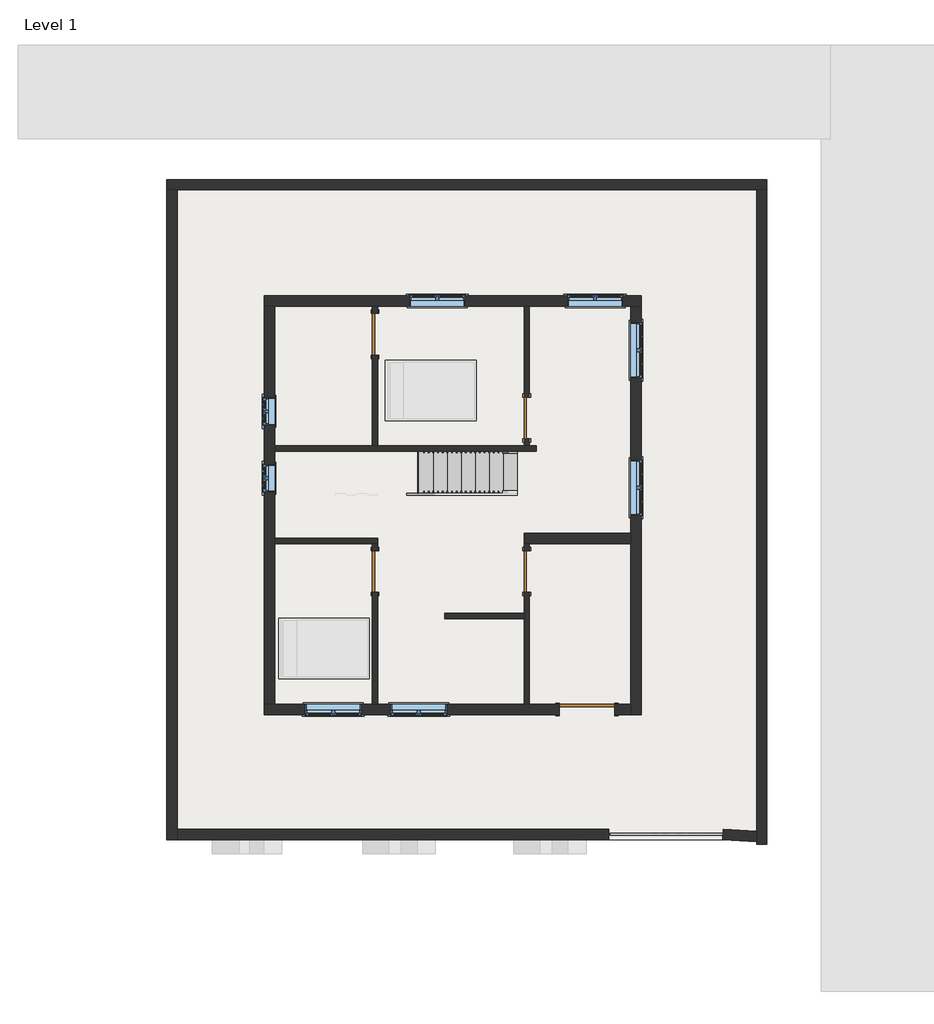
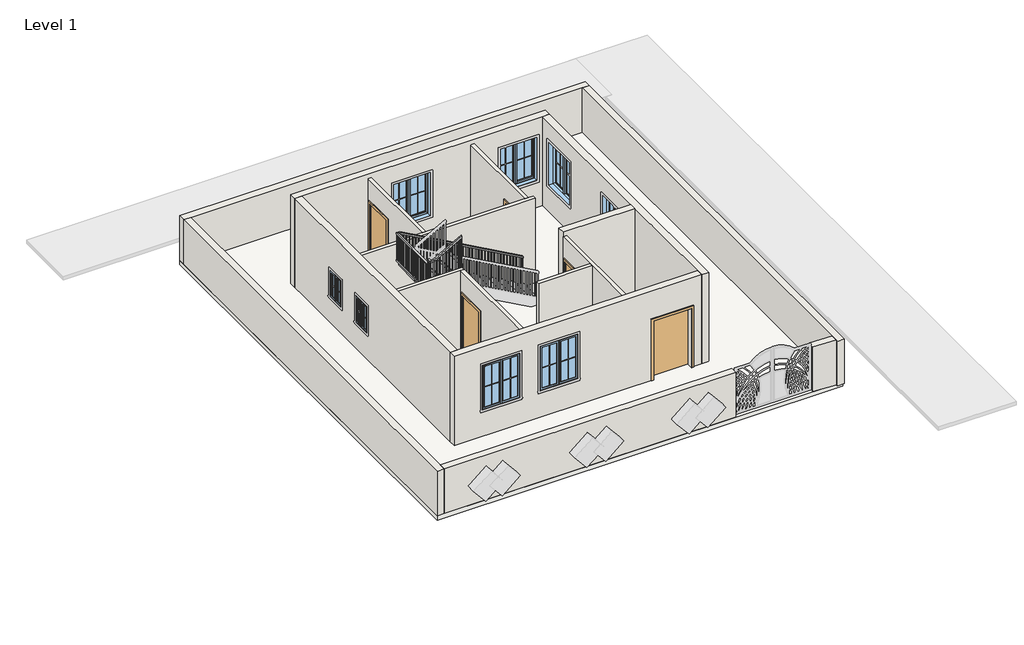
# One storey, part 1 of 2: 17 walls, 8 windows, 5 doors, 1 railing, 1 slab, 1 stair flight.
# Revit data of these elements (continued)
# Element 33 (IfcWindow, "Window-Casement-Double : 48\" x 60\"") (continued)
#   Interior Wall Closure = 0' - 2 1/4"
#   Frame Extension = 0' - 0 1/4"
#   Exterior Wall Closure = 0' - 1 1/4"
#   Interior Trim Visibility = yes
#   Exterior Trim Visibility = yes
#   Phase Created = New Construction
#   Materials on its faces: "Wood - Stained", "Glass", "Clad - White"
# Materials
#   "Door - Panel": class "Wood", colour RGB 210 159 95, transparency 0, Cost = 0
#   "Door - Frame": colour RGB 118 70 51, transparency 0, Cost = 0
#   "Softwood, Lumber": class "Wood", colour RGB 223 192 134, transparency 0, Description = "Pinus Echinata", Cost = 0
#   "Wood - Stained": class "Wood", colour RGB 224 178 126, transparency 0, Cost = 0
#   "Glass": class "Glass", colour RGB 0 128 192, transparency 0.75, Description = "Soda Lime Glass", Cost = 0
#   "Clad - White": class "Wood", colour RGB 242 242 238, transparency 0, Cost = 0
#   "Default Floor": colour RGB 128 128 128, transparency 0, Cost = 0
#   "Default Wall": colour RGB 128 128 128, transparency 0, Cost = 0
#   "Parking Stripe": class "Paint", colour RGB 250 250 91, transparency 0, Cost = 0
